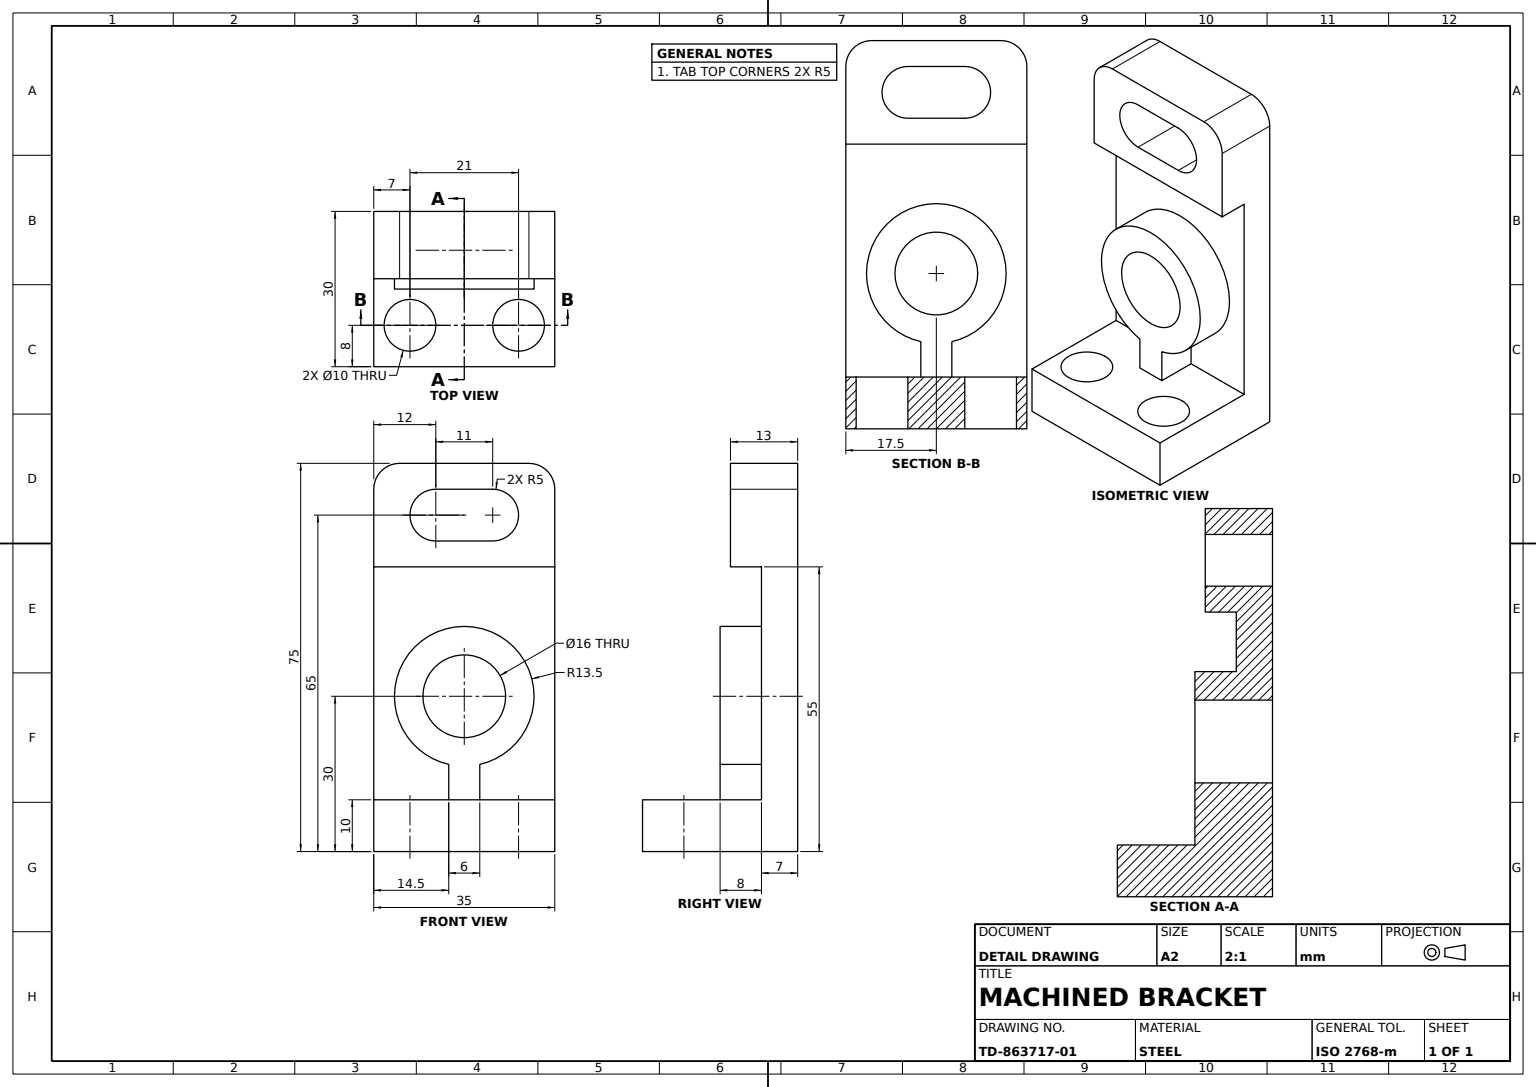
SolidWorks part; units mm, degrees
material "Plain Carbon Steel"
ref_plane "Front Plane" through (0, 0, 0) normal (0, 0, 1) x (1, 0, 0)
ref_plane "Top Plane" through (0, 0, 0) normal (0, 1, 0) x (1, 0, 0)
ref_plane "Right Plane" through (0, 0, 0) normal (1, 0, 0) x (0, 0, -1)
sketch "L Profile Sketch" plane through (0, 0, 0) normal (1, 0, 0) x (0, 0, -1)
  line L0 (0, 0) -> (-30, 0)
  line L1 (-30, 0) -> (-30, 10)
  line L2 (-30, 10) -> (-7, 10)
  line L3 (-7, 10) -> (-7, 55)
  line L4 (-7, 55) -> (-13, 55)
  line L5 (-13, 55) -> (-13, 75)
  line L6 (-13, 75) -> (0, 75)
  line L7 (0, 75) -> (0, 0)
  dimension "D1" = 20
  dimension "D2" = 10
  dimension "D3" = 30
  dimension "D4" = 13
  dimension "D5" = 7
  dimension "D6" = 55
extrude "L Bracket Body" add sketch "L Profile Sketch" along normal mid plane 35
fillet "Top Corner Fillet R5" radius 5 2 edges at (17.5, 75, 6.5) (-17.5, 75, 6.5)
sketch "Bore Boss Sketch" plane through (0, 0, 7) normal (0, 0, 1) x (1, 0, 0)
  line L0 (17.5, 10) -> (-17.5, 10) construction
  line L2 (-3, 16.8376) -> (-3, 10)
  line L3 (-3, 10) -> (3, 10)
  line L4 (3, 16.8376) -> (3, 10)
  arc A0 (3, 16.8376) -> (-3, 16.8376) centre (0, 30) ccw
  point P12 (0, 10)
  dimension "D2" = 27
  dimension "D1" = 6
  dimension "D3" = 20
extrude "Bore Boss" add sketch "Bore Boss Sketch" along normal blind 8
sketch "Bore and Slot Sketch" plane through (0, 0, 15) normal (0, 0, 1) x (1, 0, 0)
  line L0 (-5.5, 65) -> (5.5, 65) construction
  line L1 (-5.5, 70) -> (5.5, 70)
  line L2 (-5.5, 60) -> (5.5, 60)
  arc A0 (-5.5, 70) -> (-5.5, 60) centre (-5.5, 65) ccw
  arc A1 (5.5, 60) -> (5.5, 70) centre (5.5, 65) ccw
  circle A2 centre (0, 30) radius 8
  point P2 (0, 65)
  dimension "D3" = 65
  dimension "D4" = 16
  dimension "D1" = 10
  dimension "D2" = 11
extrude "Bore and Top Slot Cut" cut sketch "Bore and Slot Sketch" against normal up to surface (15 mm away) up to face at (0, 48.6785, 0)
sketch "Base Holes Sketch" plane through (0, 10, 0) normal (0, 1, 0) x (1, 0, 0)
  line L0 (0, 0) -> (0, -10.1209) construction
  line L1 (-17.5, -7) -> (-17.5, -30) construction
  line L2 (17.5, -30) -> (-17.5, -30) construction
  circle A0 centre (-10.5, -22) radius 5
  circle A1 centre (10.5, -22) radius 5
  dimension "D1" = 10
  dimension "D2" = 7
  dimension "D3" = 8
extrude "Base Mounting Holes" cut sketch "Base Holes Sketch" against normal up to surface (10 mm away) up to face at (0, 0, 15)
